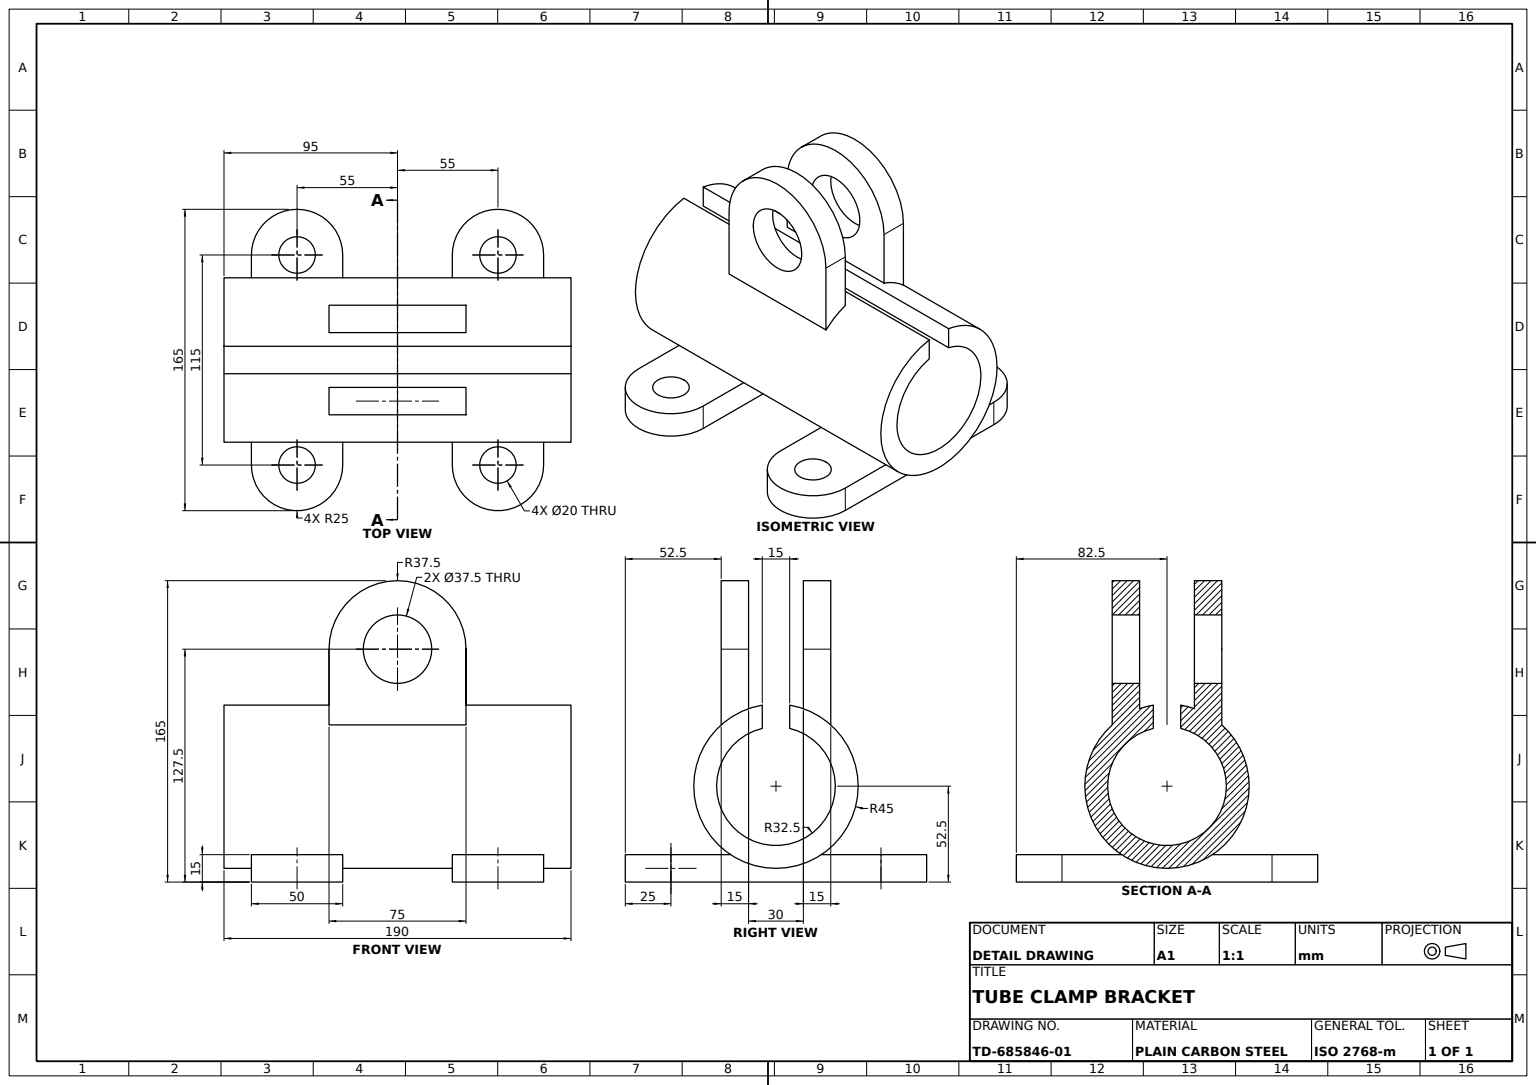
SolidWorks part; units mm, degrees
material "Plain Carbon Steel"
ref_plane "Front Plane" through (0, 0, 0) normal (0, 0, 1) x (1, 0, 0)
ref_plane "Top Plane" through (0, 0, 0) normal (0, 1, 0) x (1, 0, 0)
ref_plane "Right Plane" through (0, 0, 0) normal (1, 0, 0) x (0, 0, -1)
sketch "Split Sleeve Profile" plane through (0, 0, 0) normal (1, 0, 0) x (0, 0, -1)
  line L0 (0, 0) -> (0, 21.4548) construction
  line L1 (-7.5, 44.3706) -> (-7.5, 31.6228)
  line L2 (7.5, 44.3706) -> (7.5, 31.6228)
  arc A0 (7.5, 44.3706) -> (-7.5, 44.3706) centre (0, 0) cw
  arc A1 (7.5, 31.6228) -> (-7.5, 31.6228) centre (0, 0) cw
  dimension "D1" = 45
  dimension "D3" = 32.5
  dimension "D2" = 15
extrude "Split Sleeve" add sketch "Split Sleeve Profile" along normal mid plane 190
sketch "Saddle Base Profile" plane through (0, 0, 0) normal (0, 0, 1) x (1, 0, 0)
  line L0 (-95, -45) -> (95, -45) construction
  line L1 (-80, -37.5) -> (-30, -37.5)
  line L2 (-80, -37.5) -> (-80, -52.5)
  line L3 (-80, -52.5) -> (-30, -52.5)
  line L4 (-30, -37.5) -> (-30, -52.5)
  line L5 (-95, -45) -> (95, -45) construction
  line L6 (0, 0) -> (0, -17.7919) construction
  line L7 (30, -37.5) -> (30, -52.5)
  line L8 (80, -52.5) -> (30, -52.5)
  line L9 (80, -37.5) -> (80, -52.5)
  line L10 (80, -37.5) -> (30, -37.5)
  point P4 (-55, -37.5)
  dimension "D1" = 50
  dimension "D2" = 55
  dimension "D3" = 15
extrude "Saddle Base" add sketch "Saddle Base Profile" along normal mid plane 115
sketch "Foot Tab Profile" plane through (0, -52.5, 0) normal (0, -1, 0) x (1, 0, 0)
  line L0 (-80, 57.5) -> (-30, 57.5) construction
  line L1 (-80, 57.5) -> (-30, 57.5)
  arc A0 (-80, 57.5) -> (-30, 57.5) centre (-55, 57.5) cw
  dimension "D1" = 25
extrude "Foot Tab" add sketch "Foot Tab Profile" against normal up to surface (15 mm away) up to face at (-55, -37.5, 41.1873)
mirror "Foot Tab Mirror Front" about plane through (0, 0, 0) normal (0, 0, 1) of "Foot Tab"
mirror "Foot Tab Mirror Right" about plane through (0, 0, 0) normal (1, 0, 0) of "Foot Tab Mirror Front", "Foot Tab"
sketch "Foot Hole Profile" plane through (0, -52.5, 0) normal (0, -1, 0) x (1, 0, 0)
  circle A0 centre (-55, 57.5) radius 10
  circle A1 centre (-55, -57.5) radius 10
  circle A2 centre (55, -57.5) radius 10
  circle A3 centre (55, 57.5) radius 10
  arc A4 (-30, 57.5) -> (-80, 57.5) centre (-55, 57.5) ccw construction
  arc A5 (-80, -57.5) -> (-30, -57.5) centre (-55, -57.5) ccw construction
  arc A6 (30, -57.5) -> (80, -57.5) centre (55, -57.5) ccw construction
  arc A7 (80, 57.5) -> (30, 57.5) centre (55, 57.5) ccw construction
  dimension "D1" = 20
extrude "Foot Mounting Holes 4x" cut sketch "Foot Hole Profile" against normal up to next
ref_plane "Lug Offset Plane" through (0, 0, 15) normal (0, 0, 1) x (1, 0, 0)
sketch "Clamp Lug Profile" plane through (0, 0, 15) normal (0, 0, 1) x (1, 0, 0)
  line L0 (-37.5, 75) -> (-37.5, 31.6228)
  line L1 (-37.5, 31.6228) -> (37.5, 31.6228)
  line L2 (37.5, 31.6228) -> (37.5, 75)
  line L3 (95, 31.6228) -> (-95, 31.6228) construction
  arc A0 (-37.5, 75) -> (37.5, 75) centre (0, 75) cw
  circle A1 centre (0, 75) radius 18.75
  point P11 (0, 31.6228)
  dimension "D1" = 37.5
  dimension "D3" = 37.5
  dimension "D2" = 75
extrude "Clamp Lug" add sketch "Clamp Lug Profile" along normal blind 15
mirror "Clamp Lug Mirror" about plane through (0, 0, 0) normal (0, 0, 1) of "Clamp Lug"
